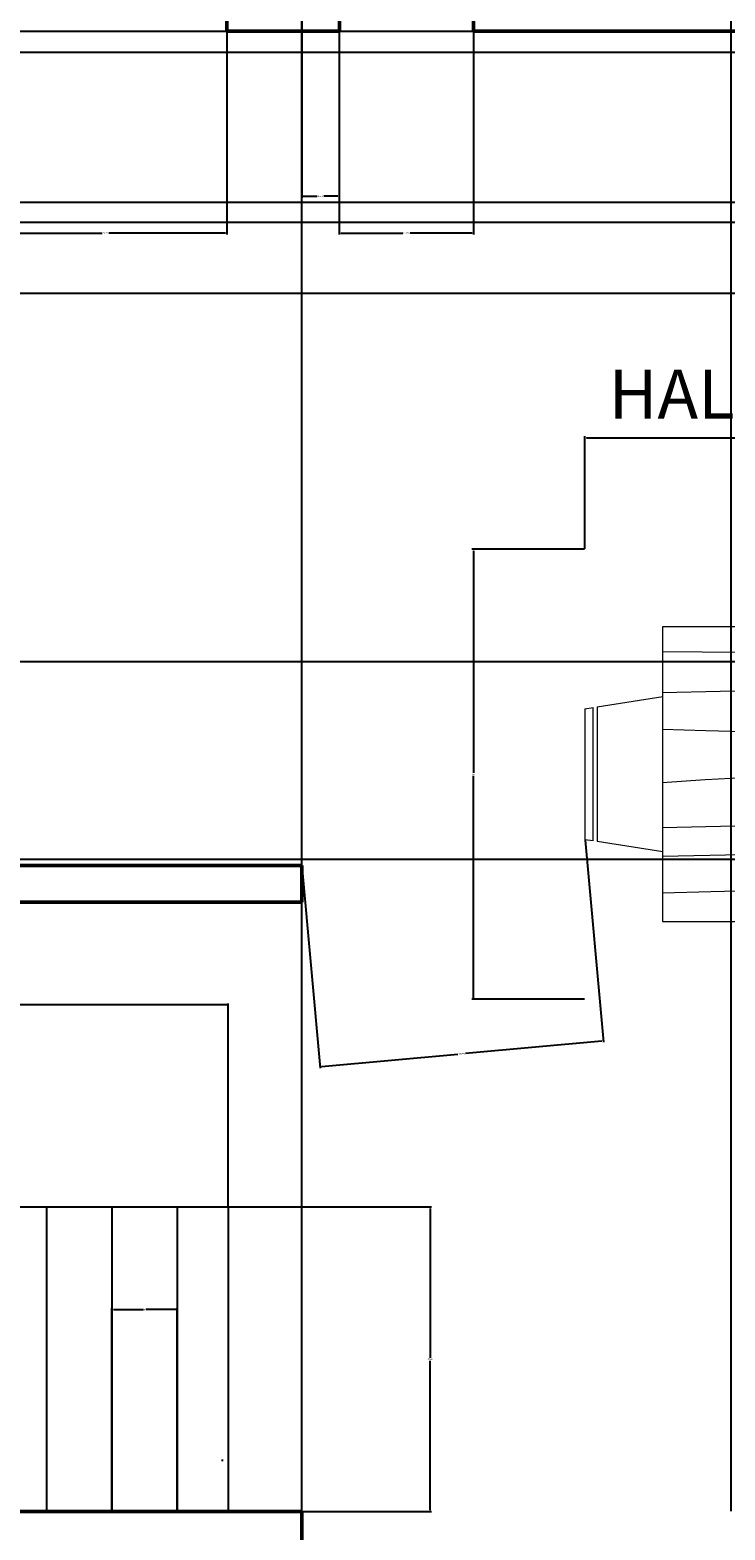
# Model space of a CAD drawing. Units: inches. Extents: x 1926 to 2293, y 1738 to 2280.
# Tile 4 of 6: x 2050 to 2135, y 1931 to 2114. Entities that reach past the tile are written whole.
import ezdxf

# ---------------------------------------------------------------- set-up
doc = ezdxf.new("R2010")
doc.units = ezdxf.units.IN
for name, color, linetype, lineweight in [('A-ANNO-DIMS', 2, 'Continuous', 18), ('A-AREA-IDEN', 7, 'Continuous', 25), ('A-FLOR-STRS', 7, 'Continuous', 25), ('A-FURN', 8, 'Continuous', 18), ('A-WALL', 7, 'Continuous', 50)]:
    doc.layers.add(name, color=color, linetype=linetype, lineweight=lineweight)
doc.styles.get("Standard").update_dxf_attribs({"font": 'arial.ttf'})
doc.dimstyles.get("Standard").update_dxf_attribs({"dimtxt": 0.18, "dimasz": 0.18, "dimexe": 0.18, "dimexo": 0.0625, "dimgap": 0.09, "dimtad": 0, "dimtih": 1, "dimtoh": 1, "dimdec": 4, "dimzin": 0, "dimdsep": 46, "dimtxsty": 'Standard', "dimcen": 0.09, "dimadec": 0, "dimazin": 0, "dimtfac": 1, "dimtdec": 4, "dimtofl": 0, "dimtmove": 0, "dimatfit": 3, "dimfxl": 1, "dimtolj": 1, "dimtzin": 0, "dimarcsym": 0})

# ---------------------------------------------------------------- blocks, each defined once
blk = doc.blocks.new('Dining Set - 36 x 72 in.')
for p, q in [((-22.2343, 26.00059), (-23.4847, 17.99762)), ((-22.2304, 26), (-5.7608, 26)), ((-22, 27.5), (-22.1562, 26.50042)), ((-5.8416, 26.5), (-22.1534, 26.5)), ((-22, 27.5), (-6, 27.5)), ((-5.8437, 26.49966), (-6, 27.5)), ((-4.5152, 17.99762), (-5.7655, 25.99926)), ((5.7657, 26.00059), (4.5153, 17.99762)), ((5.7696, 26), (22.2392, 26)), ((6, 27.5), (5.8438, 26.50042)), ((22.1584, 26.5), (5.8466, 26.5)), ((6, 27.5), (22, 27.5)), ((22.1563, 26.49966), (22, 27.5)), ((23.4848, 17.99762), (22.2345, 25.99926)), ((36, 18), (-36, 18)), ((-36, 18), (-36, -18)), ((36, -18), (36, 18)), ((-44.0006, 8.23428), (-35.9976, 9.48474)), ((44.0006, 8.23428), (35.9976, 9.48474)), ((-45.5, 8), (-44.5004, 8.15617)), ((-45.5, 8), (-45.5, -8)), ((-44.5, -8.15843), (-44.5, 8.15338)), ((-44, 8.23041), (-44, -8.23915)), ((44, 8.23041), (44, -8.23915)), ((44.5, -8.15843), (44.5, 8.15338)), ((45.5, 8), (44.5005, 8.15617)), ((45.5, 8), (45.5, -8)), ((-44.4997, -8.15631), (-45.5, -8)), ((-35.9976, -9.48476), (-43.9993, -8.2345)), ((35.9976, -9.48476), (43.9993, -8.2345)), ((44.4997, -8.15631), (45.5, -8)), ((-36, -18), (36, -18)), ((-22.2343, -26.0006), (-23.4847, -17.99762)), ((-4.5152, -17.99762), (-5.7655, -25.99928)), ((5.7657, -26.0006), (4.5153, -17.99762)), ((23.4848, -17.99762), (22.2345, -25.99928)), ((-22.2304, -26), (-5.7608, -26)), ((-22, -27.5), (-22.1562, -26.50044)), ((-5.8416, -26.5), (-22.1534, -26.5)), ((-22, -27.5), (-6, -27.5)), ((-5.8437, -26.49967), (-6, -27.5)), ((5.7696, -26), (22.2392, -26)), ((6, -27.5), (5.8438, -26.50044)), ((22.1584, -26.5), (5.8466, -26.5)), ((6, -27.5), (22, -27.5)), ((22.1563, -26.49967), (22, -27.5))]:
    blk.add_line(p, q)
for points in [[(-36, 15), (-31.1772, 14.97754), (-26.8079, 14.91406), (-22.8538, 14.81543), (-19.276, 14.6875), (-16.0362, 14.53613), (-13.0957, 14.36718), (-10.4159, 14.18652), (-7.9583, 14), (-5.6904, 13.81315), (-3.6035, 13.63021), (-1.6954, 13.45508), (0.0365, 13.29166), (1.5945, 13.14388), (2.9811, 13.01562), (4.1988, 12.9108), (5.25, 12.83333), (6.1393, 12.78613), (6.8802, 12.76823), (7.4883, 12.77767), (7.9792, 12.8125), (8.3685, 12.87077), (8.6719, 12.95052), (8.9049, 13.0498), (9.0833, 13.16666), (9.2205, 13.29899), (9.3216, 13.44401), (9.3895, 13.59879), (9.4271, 13.76041), (9.4373, 13.92594), (9.4232, 14.09245), (9.3875, 14.257), (9.3333, 14.41666), (9.2638, 14.56917), (9.1836, 14.71484), (9.0975, 14.85465), (9.0104, 14.98958), (8.9272, 15.1206), (8.8529, 15.2487), (8.7922, 15.37483), (8.75, 15.5), (8.7305, 15.62467), (8.7344, 15.74739), (8.7617, 15.86621), (8.8125, 15.97916), (8.8867, 16.08431), (8.9844, 16.17968), (9.1055, 16.26334), (9.25, 16.33333), (9.4189, 16.38802), (9.6172, 16.42708), (9.8506, 16.45052), (10.125, 16.45833), (10.4463, 16.45052), (10.8203, 16.42708), (11.2529, 16.38802), (11.75, 16.33333), (12.3184, 16.26318), (12.9694, 16.17838), (13.7151, 16.07991), (14.5677, 15.96875), (15.5395, 15.84586), (16.6426, 15.71224), (17.8893, 15.56884), (19.2917, 15.41666), (20.859, 15.25667), (22.5879, 15.08984), (24.4721, 14.91715), (26.5052, 14.73958), (28.6809, 14.5581), (30.9929, 14.3737), (33.4347, 14.18733), (36, 14)], [(-36, 10), (-28.9766, 10.14274), (-23.1725, 10.20442), (-18.4241, 10.19775), (-14.5677, 10.13541), (-11.4399, 10.03011), (-8.877, 9.89453), (-6.7154, 9.74137), (-4.7917, 9.58333), (-2.9698, 9.43082), (-1.2246, 9.28515), (0.4415, 9.14534), (2.026, 9.01041), (3.5266, 8.87939), (4.9408, 8.7513), (6.266, 8.62516), (7.5, 8.5), (8.6411, 8.37549), (9.6914, 8.2539), (10.6538, 8.13818), (11.5312, 8.03125), (12.3267, 7.93603), (13.043, 7.85547), (13.6831, 7.79248), (14.25, 7.75), (14.7471, 7.7303), (15.1797, 7.73307), (15.5537, 7.75732), (15.875, 7.80208), (16.1494, 7.86637), (16.3828, 7.94922), (16.5811, 8.04964), (16.75, 8.16666), (16.8944, 8.29915), (17.0143, 8.44531), (17.1089, 8.60319), (17.1771, 8.77083), (17.218, 8.94629), (17.2305, 9.1276), (17.2137, 9.31282), (17.1667, 9.5), (17.0895, 9.6875), (16.987, 9.875), (16.8649, 10.0625), (16.7292, 10.25), (16.5856, 10.4375), (16.4401, 10.625), (16.2985, 10.8125), (16.1667, 11), (16.05, 11.18733), (15.9518, 11.3737), (15.8752, 11.5581), (15.8229, 11.73958), (15.798, 11.91715), (15.8034, 12.08984), (15.842, 12.25667), (15.9167, 12.41666), (16.0295, 12.56836), (16.1784, 12.70833), (16.3605, 12.83268), (16.5729, 12.9375), (16.8127, 13.01888), (17.0768, 13.07291), (17.3625, 13.0957), (17.6667, 13.08333), (17.9894, 13.03312), (18.3418, 12.94726), (18.7382, 12.82918), (19.1927, 12.68229), (19.7195, 12.51001), (20.3327, 12.31575), (21.0465, 12.10294), (21.875, 11.875), (22.8357, 11.63354), (23.959, 11.37304), (25.2786, 11.08618), (26.8282, 10.76562), (28.6414, 10.40405), (30.752, 9.99414), (33.1936, 9.52856), (36, 9)], [(-36, 5.5), (-30.7157, 5.3348), (-26.069, 5.20963), (-21.9946, 5.11767), (-18.4271, 5.05208), (-15.3009, 5.00602), (-12.5508, 4.97265), (-10.1112, 4.94515), (-7.9167, 4.91666), (-5.909, 4.88167), (-4.0586, 4.83984), (-2.3429, 4.79215), (-0.7396, 4.73958), (0.7739, 4.6831), (2.22, 4.6237), (3.6213, 4.56233), (5, 4.5), (6.373, 4.43782), (7.7344, 4.3776), (9.0723, 4.32129), (10.375, 4.27083), (11.6309, 4.22819), (12.8281, 4.19531), (13.9551, 4.17415), (15, 4.16666), (15.954, 4.17448), (16.819, 4.19791), (17.6001, 4.23698), (18.3021, 4.29166), (18.9299, 4.36198), (19.4883, 4.44791), (19.9823, 4.54948), (20.4167, 4.66666), (20.7969, 4.79899), (21.1302, 4.94401), (21.4245, 5.09879), (21.6875, 5.26041), (21.9271, 5.42594), (22.1511, 5.59245), (22.3672, 5.757), (22.5834, 5.91666), (22.8065, 6.06868), (23.0404, 6.21093), (23.2879, 6.34147), (23.5521, 6.45833), (23.8358, 6.55957), (24.142, 6.64323), (24.4735, 6.70735), (24.8334, 6.75), (25.2235, 6.76969), (25.642, 6.76692), (26.0858, 6.74267), (26.5521, 6.69791), (27.0379, 6.63362), (27.5404, 6.55078), (28.0565, 6.45036), (28.5834, 6.33333), (29.1242, 6.19987), (29.7071, 6.04687), (30.3661, 5.87044), (31.1354, 5.66666), (32.0493, 5.43164), (33.142, 5.16146), (34.4475, 4.85221), (36, 4.5)], [(-36, -1), (-30.7915, -0.6591), (-26.0195, -0.38216), (-21.6519, -0.16284), (-17.6563, 0.00521), (-14.0005, 0.12833), (-10.6523, 0.21289), (-7.5796, 0.26522), (-4.75, 0.29166), (-2.134, 0.29793), (0.2878, 0.28711), (2.5317, 0.26163), (4.6146, 0.22396), (6.5529, 0.17651), (8.3633, 0.12174), (10.0623, 0.06209), (11.6667, 0), (13.1899, -0.06201), (14.6341, -0.1211), (15.9982, -0.17432), (17.2813, -0.21875), (18.4823, -0.25147), (19.6003, -0.26953), (20.6343, -0.27002), (21.5834, -0.25), (22.4481, -0.20768), (23.2357, -0.14584), (23.9549, -0.06836), (24.6146, 0.02083), (25.2235, 0.11784), (25.7904, 0.21875), (26.3241, 0.31966), (26.8334, 0.41666), (27.3265, 0.50618), (27.8099, 0.58593), (28.2894, 0.65397), (28.7709, 0.70833), (29.2601, 0.74707), (29.763, 0.76823), (30.2855, 0.76985), (30.8334, 0.75), (31.4088, 0.70784), (31.9994, 0.64713), (32.589, 0.57275), (33.1615, 0.48958), (33.7008, 0.4025), (34.1908, 0.3164), (34.6153, 0.23616), (34.9584, 0.16666), (35.2099, 0.11165), (35.3848, 0.07031), (35.504, 0.04069), (35.5886, 0.02083), (35.6594, 0.00879), (35.7377, 0.0026), (35.8442, 0.00032), (36, 0)], [(-36, -6.5), (-27.1843, -6.31267), (-20.084, -6.1263), (-14.469, -5.9419), (-10.1094, -5.76042), (-6.7752, -5.58285), (-4.2363, -5.41016), (-2.2629, -5.24333), (-0.625, -5.08334), (0.8708, -4.93099), (2.2715, -4.78646), (3.5872, -4.64974), (4.8281, -4.52084), (6.0046, -4.39974), (7.127, -4.28646), (8.2053, -4.18099), (9.25, -4.08334), (10.2705, -3.99382), (11.2734, -3.91407), (12.2647, -3.84603), (13.25, -3.79167), (14.2354, -3.75293), (15.2266, -3.73177), (16.2295, -3.73015), (17.25, -3.75), (18.2912, -3.79248), (19.3451, -3.85547), (20.4009, -3.93604), (21.4479, -4.03125), (22.4754, -4.13819), (23.4727, -4.25391), (24.4289, -4.37549), (25.3334, -4.5), (26.1785, -4.62492), (26.9694, -4.74935), (27.7145, -4.87281), (28.4219, -4.99479), (29.1, -5.11483), (29.7572, -5.23242), (30.4016, -5.34709), (31.0417, -5.45834), (31.6837, -5.56437), (32.3262, -5.65821), (32.9658, -5.73153), (33.599, -5.77604), (34.2224, -5.78345), (34.8327, -5.74545), (35.4264, -5.65373), (36, -5.5)], [(-36, -10), (-26.4022, -9.81299), (-18.4675, -9.62891), (-11.9839, -9.45069), (-6.7396, -9.28125), (-2.5226, -9.12354), (0.8789, -8.98047), (3.6769, -8.85498), (6.0833, -8.75), (8.2767, -8.66765), (10.3021, -8.60677), (12.1712, -8.56543), (13.8958, -8.54167), (15.4876, -8.53353), (16.9583, -8.53907), (18.3197, -8.55632), (19.5834, -8.58334), (20.7616, -8.61841), (21.8685, -8.66081), (22.9188, -8.71004), (23.9271, -8.76563), (24.9081, -8.82707), (25.8763, -8.89388), (26.8465, -8.96558), (27.8334, -9.04167), (28.8474, -9.12118), (29.8828, -9.20117), (30.93, -9.27824), (31.9792, -9.34896), (33.0205, -9.40991), (34.0443, -9.45768), (35.0407, -9.48885), (36, -9.5)], [(-36, -14.5), (-30.0881, -14.33513), (-25.0332, -14.21224), (-20.7312, -14.12647), (-17.0781, -14.07292), (-13.97, -14.04671), (-11.3027, -14.04297), (-8.9724, -14.05681), (-6.875, -14.08334), (-4.9224, -14.11833), (-3.0905, -14.16016), (-1.3709, -14.20785), (0.2448, -14.26042), (1.7647, -14.3169), (3.1973, -14.3763), (4.5507, -14.43767), (5.8333, -14.5), (7.0554, -14.5621), (8.235, -14.62175), (9.3922, -14.67652), (10.5469, -14.72396), (11.7192, -14.76164), (12.929, -14.78711), (14.1965, -14.79794), (15.5417, -14.79167), (16.9933, -14.76424), (18.6152, -14.70508), (20.4804, -14.60197), (22.6615, -14.44271), (25.2312, -14.21509), (28.2624, -13.9069), (31.8277, -13.50594), (36, -13)]]:
    blk.add_lwpolyline(points)
blk = doc.blocks.new('*D12')
at = {"layer": 'A-ANNO-DIMS', "color": 0, "lineweight": -2, "transparency": 16777216}
for p, q in [((2117.4, 2050.87), (2117.4, 2064.63)), ((2117.58, 2064.45), (2161.95, 2064.45)), ((2208.22, 2064.45), (2163.85, 2064.45)), ((2208.4, 2050.87), (2208.4, 2064.63))]:
    blk.add_line(p, q, dxfattribs=at)
at = {"layer": 'A-ANNO-DIMS', "color": 0, "transparency": 16777216}
for points in [[(2117.58, 2064.48), (2117.58, 2064.42), (2117.4, 2064.45)], [(2208.22, 2064.48), (2208.22, 2064.42), (2208.4, 2064.45)]]:
    blk.add_solid(points, dxfattribs=at)
at = {"layer": 'Defpoints', "color": 0, "transparency": 16777216}
for p in [(2208.4, 2064.45), (2117.4, 2050.8), (2208.4, 2050.8)]:
    blk.add_point(p, dxfattribs=at)
at = {"layer": 'A-ANNO-DIMS', "color": 0, "transparency": 16777216, "insert": (2162.9, 2064.45), "char_height": 0.18, "attachment_point": 5}
blk.add_mtext('\\A1;DINING SET 91', dxfattribs=at)
blk = doc.blocks.new('*D13')
at = {"layer": 'A-ANNO-DIMS', "color": 0, "lineweight": -2, "transparency": 16777216}
for p, q in [((2117.34, 2050.8), (2103.57, 2050.8)), ((2103.75, 2050.62), (2103.75, 2023.49)), ((2103.75, 1995.98), (2103.75, 2023.12)), ((2117.34, 1995.8), (2103.57, 1995.8))]:
    blk.add_line(p, q, dxfattribs=at)
at = {"layer": 'A-ANNO-DIMS', "color": 0, "transparency": 16777216}
for points in [[(2103.72, 2050.62), (2103.78, 2050.62), (2103.75, 2050.8)], [(2103.72, 1995.98), (2103.78, 1995.98), (2103.75, 1995.8)]]:
    blk.add_solid(points, dxfattribs=at)
at = {"layer": 'Defpoints', "color": 0, "transparency": 16777216}
for p in [(2103.75, 2050.8), (2117.4, 2050.8), (2117.4, 1995.8)]:
    blk.add_point(p, dxfattribs=at)
at = {"layer": 'A-ANNO-DIMS', "color": 0, "transparency": 16777216, "insert": (2103.75, 2023.3), "char_height": 0.18, "attachment_point": 5}
blk.add_mtext('\\A1;55', dxfattribs=at)
blk = doc.blocks.new('*D50')
at = {"layer": 'A-ANNO-DIMS', "color": 0, "lineweight": -2, "transparency": 16777216}
for p, q in [((2033.32, 2037.09), (2281.64, 2037.09)), ((2281.46, 2036.91), (2281.46, 2025.19)), ((2281.46, 2013.1), (2281.46, 2024.83)), ((2033.32, 2012.92), (2281.64, 2012.92))]:
    blk.add_line(p, q, dxfattribs=at)
at = {"layer": 'A-ANNO-DIMS', "color": 0, "transparency": 16777216}
for points in [[(2281.43, 2036.91), (2281.49, 2036.91), (2281.46, 2037.09)], [(2281.43, 2013.1), (2281.49, 2013.1), (2281.46, 2012.92)]]:
    blk.add_solid(points, dxfattribs=at)
at = {"layer": 'Defpoints', "color": 0, "transparency": 16777216}
for p in [(2033.26, 2037.09), (2281.46, 2037.09), (2033.26, 2012.92)]:
    blk.add_point(p, dxfattribs=at)
at = {"layer": 'A-ANNO-DIMS', "color": 0, "transparency": 16777216, "insert": (2281.46, 2025.01), "char_height": 0.18, "attachment_point": 5}
blk.add_mtext('\\A1;24.17', dxfattribs=at)
blk = doc.blocks.new('*D52')
at = {"layer": 'A-ANNO-DIMS', "color": 0, "lineweight": -2, "transparency": 16777216}
for p, q in [((2033.32, 2114.16), (2281.64, 2114.16)), ((2281.46, 2113.98), (2281.46, 2102.67)), ((2281.46, 2090.99), (2281.46, 2102.31)), ((2033.32, 2090.81), (2281.64, 2090.81))]:
    blk.add_line(p, q, dxfattribs=at)
at = {"layer": 'A-ANNO-DIMS', "color": 0, "transparency": 16777216}
for points in [[(2281.43, 2113.98), (2281.49, 2113.98), (2281.46, 2114.16)], [(2281.43, 2090.99), (2281.49, 2090.99), (2281.46, 2090.81)]]:
    blk.add_solid(points, dxfattribs=at)
at = {"layer": 'Defpoints', "color": 0, "transparency": 16777216}
for p in [(2033.26, 2114.16), (2281.46, 2114.16), (2033.26, 2090.81)]:
    blk.add_point(p, dxfattribs=at)
at = {"layer": 'A-ANNO-DIMS', "color": 0, "transparency": 16777216, "insert": (2281.46, 2102.49), "char_height": 0.18, "attachment_point": 5}
blk.add_mtext('\\A1;23.348', dxfattribs=at)
blk = doc.blocks.new('*D54')
at = {"layer": 'A-ANNO-DIMS', "color": 0, "lineweight": -2, "transparency": 16777216}
for p, q in [((2021.32, 2111.56), (2281.64, 2111.56)), ((2281.46, 2111.38), (2281.46, 2102.58)), ((2281.46, 2093.41), (2281.46, 2102.21)), ((2021.32, 2093.23), (2281.64, 2093.23))]:
    blk.add_line(p, q, dxfattribs=at)
at = {"layer": 'A-ANNO-DIMS', "color": 0, "transparency": 16777216}
for points in [[(2281.43, 2111.38), (2281.49, 2111.38), (2281.46, 2111.56)], [(2281.43, 2093.41), (2281.49, 2093.41), (2281.46, 2093.23)]]:
    blk.add_solid(points, dxfattribs=at)
at = {"layer": 'Defpoints', "color": 0, "transparency": 16777216}
for p in [(2021.25, 2111.56), (2281.46, 2111.56), (2021.25, 2093.23)]:
    blk.add_point(p, dxfattribs=at)
at = {"layer": 'A-ANNO-DIMS', "color": 0, "transparency": 16777216, "insert": (2281.46, 2102.39), "char_height": 0.18, "attachment_point": 5}
blk.add_mtext('\\A1;18.332', dxfattribs=at)
blk = doc.blocks.new('*D58')
at = {"layer": 'A-ANNO-DIMS', "color": 0, "lineweight": -2, "transparency": 16777216}
for p, q in [((1987.58, 2090.81), (2281.64, 2090.81)), ((2281.46, 2090.63), (2281.46, 2086.66)), ((2281.46, 2082.31), (2281.46, 2086.29)), ((1986.63, 2082.13), (2281.64, 2082.13))]:
    blk.add_line(p, q, dxfattribs=at)
at = {"layer": 'A-ANNO-DIMS', "color": 0, "transparency": 16777216}
for points in [[(2281.43, 2090.63), (2281.49, 2090.63), (2281.46, 2090.81)], [(2281.43, 2082.31), (2281.49, 2082.31), (2281.46, 2082.13)]]:
    blk.add_solid(points, dxfattribs=at)
at = {"layer": 'Defpoints', "color": 0, "transparency": 16777216}
for p in [(1987.52, 2090.81), (2281.46, 2090.81), (1986.57, 2082.13)]:
    blk.add_point(p, dxfattribs=at)
at = {"layer": 'A-ANNO-DIMS', "color": 0, "transparency": 16777216, "insert": (2281.46, 2086.47), "char_height": 0.18, "attachment_point": 5}
blk.add_mtext('\\A1;8.682', dxfattribs=at)
blk = doc.blocks.new('*D59')
at = {"layer": 'A-ANNO-DIMS', "color": 0, "lineweight": -2, "transparency": 16777216}
for p, q in [((2082.76, 2118.6), (2082.76, 2093.78)), ((2087.35, 2118.6), (2087.35, 2093.78)), ((2082.94, 2093.96), (2084.66, 2093.96)), ((2087.17, 2093.96), (2085.45, 2093.96))]:
    blk.add_line(p, q, dxfattribs=at)
at = {"layer": 'A-ANNO-DIMS', "color": 0, "transparency": 16777216}
for points in [[(2082.94, 2093.99), (2082.94, 2093.93), (2082.76, 2093.96)], [(2087.17, 2093.99), (2087.17, 2093.93), (2087.35, 2093.96)]]:
    blk.add_solid(points, dxfattribs=at)
at = {"layer": 'Defpoints', "color": 0, "transparency": 16777216}
for p in [(2082.76, 2118.66), (2087.35, 2118.66), (2082.76, 2093.96)]:
    blk.add_point(p, dxfattribs=at)
at = {"layer": 'A-ANNO-DIMS', "color": 0, "transparency": 16777216, "insert": (2085.05, 2093.96), "char_height": 0.18, "attachment_point": 5}
blk.add_mtext('\\A1;4.595', dxfattribs=at)
blk = doc.blocks.new('*D60')
at = {"layer": 'A-ANNO-DIMS', "color": 0, "lineweight": -2, "transparency": 16777216}
for p, q in [((2087.35, 2114.1), (2087.35, 2089.28)), ((2103.76, 2114.1), (2103.76, 2089.28)), ((2087.53, 2089.46), (2095.1, 2089.46)), ((2103.58, 2089.46), (2096.01, 2089.46))]:
    blk.add_line(p, q, dxfattribs=at)
at = {"layer": 'A-ANNO-DIMS', "color": 0, "transparency": 16777216}
for points in [[(2087.53, 2089.49), (2087.53, 2089.43), (2087.35, 2089.46)], [(2103.58, 2089.49), (2103.58, 2089.43), (2103.76, 2089.46)]]:
    blk.add_solid(points, dxfattribs=at)
at = {"layer": 'Defpoints', "color": 0, "transparency": 16777216}
for p in [(2087.35, 2114.16), (2103.76, 2114.16), (2087.35, 2089.46)]:
    blk.add_point(p, dxfattribs=at)
at = {"layer": 'A-ANNO-DIMS', "color": 0, "transparency": 16777216, "insert": (2095.55, 2089.46), "char_height": 0.18, "attachment_point": 5}
blk.add_mtext('\\A1;16.405', dxfattribs=at)
blk = doc.blocks.new('*D61')
at = {"layer": 'A-ANNO-DIMS', "color": 0, "lineweight": -2, "transparency": 16777216}
for p, q in [((2082.76, 1933.22), (2082.76, 2280.04)), ((2082.94, 2279.86), (2108.63, 2279.86)), ((2135.12, 2279.86), (2109.42, 2279.86)), ((2135.3, 1933.22), (2135.3, 2280.04))]:
    blk.add_line(p, q, dxfattribs=at)
at = {"layer": 'A-ANNO-DIMS', "color": 0, "transparency": 16777216}
for points in [[(2082.94, 2279.89), (2082.94, 2279.83), (2082.76, 2279.86)], [(2135.12, 2279.89), (2135.12, 2279.83), (2135.3, 2279.86)]]:
    blk.add_solid(points, dxfattribs=at)
at = {"layer": 'Defpoints', "color": 0, "transparency": 16777216}
for p in [(2135.3, 2279.86), (2082.76, 1933.16), (2135.3, 1933.16)]:
    blk.add_point(p, dxfattribs=at)
at = {"layer": 'A-ANNO-DIMS', "color": 0, "transparency": 16777216, "insert": (2109.03, 2279.86), "char_height": 0.18, "attachment_point": 5}
blk.add_mtext('\\A1;52.54', dxfattribs=at)
blk = doc.blocks.new('*D63')
at = {"layer": 'A-ANNO-DIMS', "color": 0, "lineweight": -2, "transparency": 16777216}
for p, q in [((2043.88, 2114.1), (2043.88, 2089.28)), ((2073.61, 2114.1), (2073.61, 2089.28)), ((2044.06, 2089.46), (2058.35, 2089.46)), ((2073.43, 2089.46), (2059.14, 2089.46))]:
    blk.add_line(p, q, dxfattribs=at)
at = {"layer": 'A-ANNO-DIMS', "color": 0, "transparency": 16777216}
for points in [[(2044.06, 2089.49), (2044.06, 2089.43), (2043.88, 2089.46)], [(2073.43, 2089.49), (2073.43, 2089.43), (2073.61, 2089.46)]]:
    blk.add_solid(points, dxfattribs=at)
at = {"layer": 'Defpoints', "color": 0, "transparency": 16777216}
for p in [(2043.88, 2114.16), (2073.61, 2114.16), (2043.88, 2089.46)]:
    blk.add_point(p, dxfattribs=at)
at = {"layer": 'A-ANNO-DIMS', "color": 0, "transparency": 16777216, "insert": (2058.74, 2089.46), "char_height": 0.18, "attachment_point": 5}
blk.add_mtext('\\A1;29.73', dxfattribs=at)
blk = doc.blocks.new('*D67')
at = {"layer": 'A-ANNO-DIMS', "color": 0, "lineweight": -2, "transparency": 16777216}
for p, q in [((2059.53, 1933.22), (2059.53, 1958.04)), ((2059.71, 1957.86), (2063.38, 1957.86)), ((2067.35, 1957.86), (2063.68, 1957.86)), ((2067.53, 1933.22), (2067.53, 1958.04))]:
    blk.add_line(p, q, dxfattribs=at)
at = {"layer": 'A-ANNO-DIMS', "color": 0, "transparency": 16777216}
for points in [[(2059.71, 1957.89), (2059.71, 1957.83), (2059.53, 1957.86)], [(2067.35, 1957.89), (2067.35, 1957.83), (2067.53, 1957.86)]]:
    blk.add_solid(points, dxfattribs=at)
at = {"layer": 'Defpoints', "color": 0, "transparency": 16777216}
for p in [(2067.53, 1957.86), (2059.53, 1933.16), (2067.53, 1933.16)]:
    blk.add_point(p, dxfattribs=at)
at = {"layer": 'A-ANNO-DIMS', "color": 0, "transparency": 16777216, "insert": (2063.53, 1957.86), "char_height": 0.18, "attachment_point": 5}
blk.add_mtext('\\A1;8', dxfattribs=at)
blk = doc.blocks.new('*D69')
at = {"layer": 'A-ANNO-DIMS', "color": 0, "lineweight": -2, "transparency": 16777216}
for p, q in [((1987.53, 1970.47), (1987.53, 1995.29)), ((2073.75, 1970.47), (2073.75, 1995.29)), ((1987.71, 1995.11), (2030.25, 1995.11)), ((2073.57, 1995.11), (2031.03, 1995.11))]:
    blk.add_line(p, q, dxfattribs=at)
at = {"layer": 'A-ANNO-DIMS', "color": 0, "transparency": 16777216}
for points in [[(1987.71, 1995.14), (1987.71, 1995.08), (1987.53, 1995.11)], [(2073.57, 1995.14), (2073.57, 1995.08), (2073.75, 1995.11)]]:
    blk.add_solid(points, dxfattribs=at)
at = {"layer": 'Defpoints', "color": 0, "transparency": 16777216}
for p in [(2073.75, 1995.11), (1987.53, 1970.41), (2073.75, 1970.41)]:
    blk.add_point(p, dxfattribs=at)
at = {"layer": 'A-ANNO-DIMS', "color": 0, "transparency": 16777216, "insert": (2030.64, 1995.11), "char_height": 0.18, "attachment_point": 5}
blk.add_mtext('\\A1;86.22', dxfattribs=at)
blk = doc.blocks.new('*D70')
at = {"layer": 'A-ANNO-DIMS', "color": 0, "lineweight": -2, "transparency": 16777216}
for p, q in [((2073.81, 1970.41), (2098.63, 1970.41)), ((2098.45, 1970.23), (2098.45, 1951.97)), ((2098.45, 1933.34), (2098.45, 1951.61)), ((2073.81, 1933.16), (2098.63, 1933.16))]:
    blk.add_line(p, q, dxfattribs=at)
at = {"layer": 'A-ANNO-DIMS', "color": 0, "transparency": 16777216}
for points in [[(2098.42, 1970.23), (2098.48, 1970.23), (2098.45, 1970.41)], [(2098.42, 1933.34), (2098.48, 1933.34), (2098.45, 1933.16)]]:
    blk.add_solid(points, dxfattribs=at)
at = {"layer": 'Defpoints', "color": 0, "transparency": 16777216}
for p in [(2073.75, 1970.41), (2073.75, 1933.16), (2098.45, 1933.16)]:
    blk.add_point(p, dxfattribs=at)
at = {"layer": 'A-ANNO-DIMS', "color": 0, "transparency": 16777216, "insert": (2098.45, 1951.79), "char_height": 0.18, "attachment_point": 5}
blk.add_mtext('\\A1;37.25', dxfattribs=at)
blk = doc.blocks.new('*D81')
at = {"layer": 'A-ANNO-DIMS', "color": 0, "lineweight": -2, "transparency": 16777216}
for p, q in [((2117.41, 2015.24), (2119.65, 1990.53)), ((2082.76, 2012.1), (2085, 1987.38)), ((2119.45, 1990.69), (2102.77, 1989.18)), ((2085.17, 1987.58), (2101.85, 1989.09))]:
    blk.add_line(p, q, dxfattribs=at)
at = {"layer": 'A-ANNO-DIMS', "color": 0, "transparency": 16777216}
for points in [[(2119.45, 1990.72), (2119.45, 1990.66), (2119.63, 1990.71)], [(2085.16, 1987.61), (2085.17, 1987.55), (2084.99, 1987.56)]]:
    blk.add_solid(points, dxfattribs=at)
at = {"layer": 'Defpoints', "color": 0, "transparency": 16777216}
for p in [(2117.4, 2015.3), (2082.76, 2012.16), (2084.99, 1987.56)]:
    blk.add_point(p, dxfattribs=at)
at = {"layer": 'A-ANNO-DIMS', "color": 0, "transparency": 16777216, "insert": (2102.31, 1989.13), "char_height": 0.18, "attachment_point": 5}
blk.add_mtext('\\A1;34.785', dxfattribs=at)
blk = doc.blocks.new('*D88')
at = {"layer": 'A-ANNO-DIMS', "color": 0, "lineweight": -2, "transparency": 16777216}
for p, q in [((2072.97, 1939.43), (2073.15, 1939.43)), ((2073.06, 1939.34), (2073.06, 1939.52)), ((2043.15, 1883.11), (2054.28, 1904.07)), ((2042.97, 1883.11), (2043.15, 1883.11))]:
    blk.add_line(p, q, dxfattribs=at)
at = {"layer": 'A-ANNO-DIMS', "color": 0, "transparency": 16777216}
blk.add_solid([(2054.26, 1904.08), (2054.31, 1904.06), (2054.37, 1904.23)], dxfattribs=at)
at = {"layer": 'Defpoints', "color": 0, "transparency": 16777216}
for p in [(2073.06, 1939.43), (2054.37, 1904.23)]:
    blk.add_point(p, dxfattribs=at)
at = {"layer": 'A-ANNO-DIMS', "color": 0, "transparency": 16777216, "insert": (2042.49, 1883.11), "char_height": 0.18, "attachment_point": 5}
blk.add_mtext('\\A1;R39.85', dxfattribs=at)

msp = doc.modelspace()

# ---------------------------------------------------------------- linework, layer by layer
at = {"layer": 'A-FLOR-STRS'}
for p, q in [((1987.531, 1970.4122), (2073.7521, 1970.4122)), ((2051.531, 1970.4122), (2051.531, 1933.1622)), ((2059.531, 1970.4122), (2059.531, 1933.1622)), ((2067.531, 1970.4122), (2067.531, 1933.1622)), ((2073.7521, 1970.4122), (2073.7521, 1933.1622))]:
    msp.add_line(p, q, dxfattribs=at)
at = {"layer": 'A-WALL'}
for p, q in [((2073.6065, 2114.1622), (2073.6065, 2118.6622)), ((2087.3518, 2114.1622), (2087.3518, 2118.6622)), ((2103.7569, 2114.1622), (2103.7569, 2118.6622)), ((2073.6065, 2114.1622), (2087.3518, 2114.1622)), ((2103.7569, 2114.1622), (2141.6268, 2114.1622)), ((2037.7569, 2012.1622), (2082.7569, 2012.1622)), ((2082.7569, 2012.1622), (2082.7569, 2007.6622)), ((2037.7569, 2007.6622), (2078.2569, 2007.6622)), ((2078.2569, 2007.6622), (2082.7569, 2007.6622)), ((2082.7569, 1933.1622), (1959.7569, 1933.1622)), ((2082.7569, 1933.1622), (2082.7569, 1928.6622)), ((2082.7569, 1933.1622), (2082.7569, 1928.6622))]:
    msp.add_line(p, q, dxfattribs=at)

# ---------------------------------------------------------------- block references
at = {"layer": 'A-FURN'}
msp.add_blockref('Dining Set - 36 x 72 in.', (2162.8994, 2023.3046), dxfattribs=at)

# ---------------------------------------------------------------- texts
at = {"layer": 'A-AREA-IDEN', "insert": (2120.3037, 2072.7791), "char_height": 6, "attachment_point": 1}
msp.add_mtext_dynamic_manual_height_columns('HALL +DINING AREA', width=89.283239, gutter_width=12.5, heights=[0], dxfattribs=at)

# ---------------------------------------------------------------- dimensions: what is measured, and where the dimension line sits
at = {"layer": 'A-ANNO-DIMS'}
for base, p1, p2, override, picture, middle in [((2135.2979, 2279.8622), (2082.7569, 1933.1622), (2135.2979, 1933.1622), {"dimdec": 2, "dimlfac": 1, "dimrnd": 0, "dimzin": 0, "dimdsep": 46, "dimlunit": 2}, '*D61', (2109.0274, 2279.8622)), ((2073.7521, 1995.1122), (1987.531, 1970.4122), (2073.7521, 1970.4122), {"dimdec": 2, "dimlfac": 1, "dimrnd": 0, "dimzin": 0, "dimdsep": 46, "dimlunit": 2}, '*D69', (2030.6415, 1995.1122)), ((2067.531, 1957.8622), (2059.531, 1933.1622), (2067.531, 1933.1622), {"dimdec": 0, "dimlfac": 1, "dimrnd": 0, "dimzin": 0, "dimdsep": 46, "dimlunit": 2}, '*D67', (2063.531, 1957.8622))]:
    dim = msp.add_linear_dim(base=base, p1=p1, p2=p2, dimstyle='Standard', override=override, dxfattribs=at)
    dim.commit()
    dim.dimension.update_dxf_attribs({"geometry": picture, "text_midpoint": middle})
for base, p1, p2, angle, override, picture, middle in [((2082.7569, 2093.9622), (2087.3518, 2118.6622), (2082.7569, 2118.6622), 180, {"dimdec": 3, "dimlfac": 1, "dimrnd": 0, "dimzin": 0, "dimdsep": 46, "dimlunit": 2}, '*D59', (2085.0543, 2093.9622)), ((2281.4569, 2114.1622), (2033.2569, 2090.8146), (2033.2569, 2114.1622), 90, {"dimdec": 3, "dimlfac": 1, "dimrnd": 0, "dimzin": 0, "dimdsep": 46, "dimlunit": 2}, '*D52', (2281.4569, 2102.4884)), ((2043.8774, 2089.4622), (2073.6065, 2114.1622), (2043.8774, 2114.1622), 180, {"dimdec": 2, "dimlfac": 1, "dimrnd": 0, "dimzin": 0, "dimdsep": 46, "dimlunit": 2}, '*D63', (2058.7419, 2089.4622)), ((2087.3518, 2089.4622), (2103.7569, 2114.1622), (2087.3518, 2114.1622), 180, {"dimdec": 3, "dimlfac": 1, "dimrnd": 0, "dimzin": 0, "dimdsep": 46, "dimlunit": 2}, '*D60', (2095.5543, 2089.4622)), ((2281.4569, 2111.5596), (2021.2546, 2093.2275), (2021.2546, 2111.5596), 90, {"dimdec": 3, "dimlfac": 1, "dimrnd": 0, "dimzin": 0, "dimdsep": 46, "dimlunit": 2}, '*D54', (2281.4569, 2102.3935)), ((2281.4569, 2090.8146), (1986.5655, 2082.133), (1987.5186, 2090.8146), 90, {"dimdec": 3, "dimlfac": 1, "dimrnd": 0, "dimzin": 0, "dimdsep": 46, "dimlunit": 2}, '*D58', (2281.4569, 2086.4738)), ((2103.7494, 2050.8046), (2117.3994, 1995.8046), (2117.3994, 2050.8046), 90, {"dimdec": 0, "dimlfac": 1, "dimrnd": 0, "dimzin": 0, "dimdsep": 46, "dimlunit": 2}, '*D13', (2103.7494, 2023.3046)), ((2281.4569, 2037.0927), (2033.2569, 2012.9217), (2033.2569, 2037.0927), 90, {"dimdec": 2, "dimlfac": 1, "dimrnd": 0, "dimzin": 0, "dimdsep": 46, "dimlunit": 2}, '*D50', (2281.4569, 2025.0072)), ((2084.9882, 1987.5632), (2117.3994, 2015.3046), (2082.7569, 2012.1622), 185.183004, {"dimdec": 3, "dimlfac": 1, "dimrnd": 0, "dimzin": 0, "dimdsep": 46, "dimlunit": 2}, '*D81', (2102.3095, 1989.1344)), ((2098.4521, 1933.1622), (2073.7521, 1970.4122), (2073.7521, 1933.1622), 270, {"dimdec": 2, "dimlfac": 1, "dimrnd": 0, "dimzin": 0, "dimdsep": 46, "dimlunit": 2}, '*D70', (2098.4521, 1951.7872))]:
    dim = msp.add_linear_dim(base=base, p1=p1, p2=p2, angle=angle, dimstyle='Standard', override=override, dxfattribs=at)
    dim.commit()
    dim.dimension.update_dxf_attribs({"geometry": picture, "text_midpoint": middle})
dim = msp.add_linear_dim(base=(2208.3994, 2064.4546), p1=(2117.3994, 2050.8046), p2=(2208.3994, 2050.8046), text='DINING SET <>', dimstyle='Standard', override={"dimdec": 0, "dimlfac": 1, "dimrnd": 0, "dimzin": 0, "dimdsep": 46, "dimlunit": 2}, dxfattribs=at)
dim.commit()
dim.dimension.update_dxf_attribs({"geometry": '*D12', "text_midpoint": (2162.8994, 2064.4546)})
dim = msp.add_radius_dim(center=(2073.0583, 1939.4257), mpoint=(2054.3671, 1904.2282), dimstyle='Standard', override={"dimdec": 2, "dimlfac": 1, "dimrnd": 0, "dimzin": 0, "dimdsep": 46, "dimlunit": 2}, dxfattribs=at)
dim.commit()
dim.dimension.update_dxf_attribs({"geometry": '*D88', "text_midpoint": (2042.4919, 1883.1098), "dimtype": 164})

doc.saveas('drawing.dxf')
